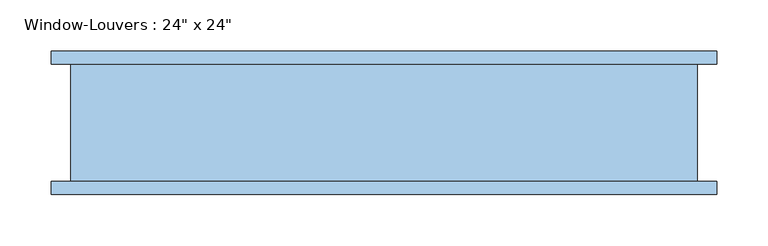
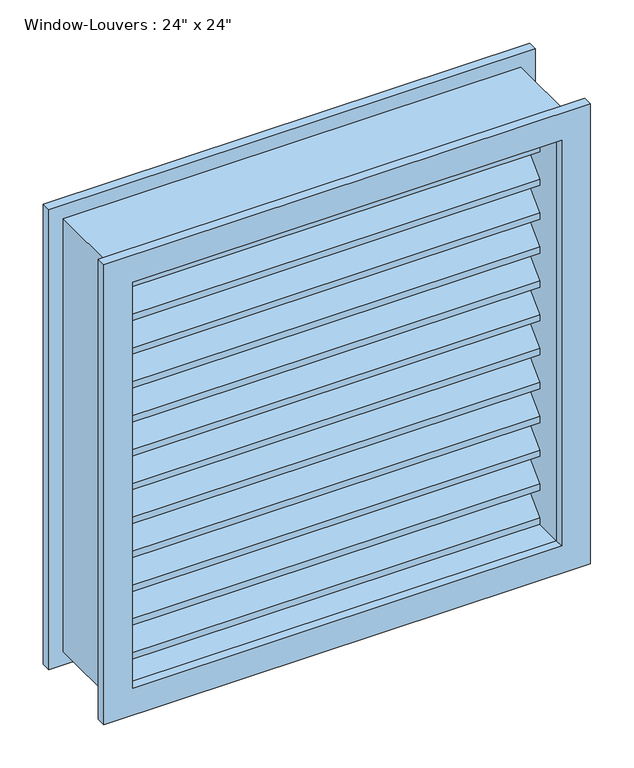
"""IFC4 building model written with IfcOpenShell, lengths in millimetres: window geometry."""

from ifc_helpers import new_model, si_unit, frame, origin, place, context, project, spatial, polyline, outline, extrude, source, transform, mapped, element, save


def window_d39e7ecb(model_context):
    return source(origin(), model_context, "Body", "SweptSolid", [
        extrude(outline(polyline([(50.8, 1419.1754778), (50.8, 1410.1952217), (12.7, 1448.2952217), (-25.4, 1410.1952217), (-25.4, 1419.1754778), (12.7, 1457.2754778), (50.8, 1419.1754778)])), frame((-285.75, 0.0, 0.0), z_axis=(1.0, 0.0, 0.0), x_axis=(0.0, 1.0, 0.0)), (0.0, 0.0, 1.0), 571.5),
        extrude(outline(polyline([(50.8, 1371.5009557), (50.8, 1362.5206995), (12.7, 1400.6206995), (-25.4, 1362.5206995), (-25.4, 1371.5009557), (12.7, 1409.6009557), (50.8, 1371.5009557)])), frame((-285.75, 0.0, 0.0), z_axis=(1.0, 0.0, 0.0), x_axis=(0.0, 1.0, 0.0)), (0.0, 0.0, 1.0), 571.5),
        extrude(outline(polyline([(50.8, 1323.8264335), (50.8, 1314.8461774), (12.7, 1352.9461774), (-25.4, 1314.8461774), (-25.4, 1323.8264335), (12.7, 1361.9264335), (50.8, 1323.8264335)])), frame((-285.75, 0.0, 0.0), z_axis=(1.0, 0.0, 0.0), x_axis=(0.0, 1.0, 0.0)), (0.0, 0.0, 1.0), 571.5),
        extrude(outline(polyline([(50.8, 1276.1519113), (50.8, 1267.1716552), (12.7, 1305.2716552), (-25.4, 1267.1716552), (-25.4, 1276.1519113), (12.7, 1314.2519113), (50.8, 1276.1519113)])), frame((-285.75, 0.0, 0.0), z_axis=(1.0, 0.0, 0.0), x_axis=(0.0, 1.0, 0.0)), (0.0, 0.0, 1.0), 571.5),
        extrude(outline(polyline([(50.8, 1228.4773891), (50.8, 1219.497133), (12.7, 1257.597133), (-25.4, 1219.497133), (-25.4, 1228.4773891), (12.7, 1266.5773891), (50.8, 1228.4773891)])), frame((-285.75, 0.0, 0.0), z_axis=(1.0, 0.0, 0.0), x_axis=(0.0, 1.0, 0.0)), (0.0, 0.0, 1.0), 571.5),
        extrude(outline(polyline([(50.8, 1180.802867), (50.8, 1171.8226109), (12.7, 1209.9226109), (-25.4, 1171.8226109), (-25.4, 1180.802867), (12.7, 1218.902867), (50.8, 1180.802867)])), frame((-285.75, 0.0, 0.0), z_axis=(1.0, 0.0, 0.0), x_axis=(0.0, 1.0, 0.0)), (0.0, 0.0, 1.0), 571.5),
        extrude(outline(polyline([(50.8, 1133.1283448), (50.8, 1124.1480887), (12.7, 1162.2480887), (-25.4, 1124.1480887), (-25.4, 1133.1283448), (12.7, 1171.2283448), (50.8, 1133.1283448)])), frame((-285.75, 0.0, 0.0), z_axis=(1.0, 0.0, 0.0), x_axis=(0.0, 1.0, 0.0)), (0.0, 0.0, 1.0), 571.5),
        extrude(outline(polyline([(50.8, 1085.4538226), (50.8, 1076.4735665), (12.7, 1114.5735665), (-25.4, 1076.4735665), (-25.4, 1085.4538226), (12.7, 1123.5538226), (50.8, 1085.4538226)])), frame((-285.75, 0.0, 0.0), z_axis=(1.0, 0.0, 0.0), x_axis=(0.0, 1.0, 0.0)), (0.0, 0.0, 1.0), 571.5),
        extrude(outline(polyline([(50.8, 1037.7793005), (50.8, 1028.7990443), (12.7, 1066.8990443), (-25.4, 1028.7990443), (-25.4, 1037.7793005), (12.7, 1075.8793005), (50.8, 1037.7793005)])), frame((-285.75, 0.0, 0.0), z_axis=(1.0, 0.0, 0.0), x_axis=(0.0, 1.0, 0.0)), (0.0, 0.0, 1.0), 571.5),
        extrude(outline(polyline([(50.8, 990.1047783), (50.8, 981.1245222), (12.7, 1019.2245222), (-25.4, 981.1245222), (-25.4, 990.1047783), (12.7, 1028.2047783), (50.8, 990.1047783)])), frame((-285.75, 0.0, 0.0), z_axis=(1.0, 0.0, 0.0), x_axis=(0.0, 1.0, 0.0)), (0.0, 0.0, 1.0), 571.5),
        extrude(outline(polyline([(50.8, 1466.85), (50.8, 1457.8697439), (12.7, 1495.9697439), (-25.4, 1457.8697439), (-25.4, 1466.85), (12.7, 1504.95), (50.8, 1466.85)])), frame((-285.75, 0.0, 0.0), z_axis=(1.0, 0.0, 0.0), x_axis=(0.0, 1.0, 0.0)), (0.0, 0.0, 1.0), 571.5),
        extrude(outline(polyline([(50.8, 942.4302561), (50.8, 933.45), (12.7, 971.55), (-25.4, 933.45), (-25.4, 942.4302561), (12.7, 980.5302561), (50.8, 942.4302561)])), frame((-285.75, 0.0, 0.0), z_axis=(1.0, 0.0, 0.0), x_axis=(0.0, 1.0, 0.0)), (0.0, 0.0, 1.0), 571.5),
        extrude(outline(polyline([(1524.0, 304.8), (1524.0, -304.8), (914.4, -304.8), (914.4, 304.8), (1524.0, 304.8)]), holes=[polyline([(1504.95, 285.75), (933.45, 285.75), (933.45, -285.75), (1504.95, -285.75), (1504.95, 285.75)])]), frame((0.0, -63.5, 0.0), z_axis=(0.0, 1.0, 0.0), x_axis=(0.0, 0.0, 1.0)), (0.0, 0.0, 1.0), 114.3),
        extrude(outline(polyline([(1543.05, 323.85), (1543.05, -323.85), (895.35, -323.85), (895.35, 323.85), (1543.05, 323.85)]), holes=[polyline([(1504.95, 285.75), (933.45, 285.75), (933.45, -285.75), (1504.95, -285.75), (1504.95, 285.75)])]), frame((0.0, -76.2, 0.0), z_axis=(0.0, 1.0, 0.0), x_axis=(0.0, 0.0, 1.0)), (0.0, 0.0, 1.0), 12.7),
        extrude(outline(polyline([(1543.05, -323.85), (895.35, -323.85), (895.35, 323.85), (1543.05, 323.85), (1543.05, -323.85)]), holes=[polyline([(1504.95, -285.75), (1504.95, 285.75), (933.45, 285.75), (933.45, -285.75), (1504.95, -285.75)])]), frame((0.0, 50.8, 0.0), z_axis=(0.0, 1.0, 0.0), x_axis=(0.0, 0.0, 1.0)), (0.0, 0.0, 1.0), 12.7),
    ])


if __name__ == "__main__":
    model = new_model("IFC4")
    model_context = context("Model", 3, world=origin())
    ifc_project = project(units=[si_unit("LENGTHUNIT", "METRE", prefix="MILLI")], contexts=[model_context])
    site = spatial("IfcSite", under=ifc_project)
    building = spatial("IfcBuilding", under=site)
    placement = place(None, origin())
    window_shape = window_d39e7ecb(model_context)
    element("IfcWindow", 1, ObjectType="Window-Louvers : 24\" x 24\"", at=placement, inside=building, context=model_context, shape_type="MappedRepresentation", body=[
        mapped(window_shape, transform((0.0, 0.0, 0.0), x_axis=(1.0, 0.0, 0.0), y_axis=(0.0, 1.0, 0.0), z_axis=(0.0, 0.0, 1.0))),
    ])
    save(model, "model.ifc")

# Revit data of these elements
# Type "Window-Louvers : 24\" x 24\""
#   Type Mark = "26"
#   Construction Type Id = "GSP4R"
#   Assembly Code = "B20"
#   Analytic Construction = "1/8 in Pilkington single glazing"
#   Visual Light Transmittance = 0.9
#   Thermal Resistance (R) = 1.53941 (h·ft²·°F)/BTU
#   Solar Heat Gain Coefficient = 0.78
#   Max Height = 1.978553 ft
#   Height = 2 ft
#   Heat Transfer Coefficient (U) = 0.6496 BTU/(h·ft²·°F)
#   Blade Width [instance default] = 1.875 ft
#   Blade Vertical Thickness = 0.029463 ft
#   Blade Thickness = 0.020833 ft
#   Blade Spacing = 0.125 ft
#   Blade Height = 0.154463 ft
#   Blade Depth = 0.25 ft
#   Blade Angle = 45.00°
#   Default Sill Height = 3 ft
#   Trim Projection_Exterior = 0.041667 ft
#   Trim Projection_Interior = 0.041667 ft
#   Trim Width_Exterior = 0.125 ft
#   Trim Width_Interior = 0.125 ft
#   Width = 2 ft
#   Max Blade Count = 12
#   Define Thermal Properties by = 1
#   Blade Count = 12
#   Frame Material = Birch
#   Louver Material = Birch
#   Trim Exterior Material = Birch
#   Trim Interior Material = Birch
#   Wall Closure = (empty or 0)
# Element 1 (IfcWindow, "Window-Louvers : 24\" x 24\"")
#   Materials on its faces: "Birch"
# Materials
#   "Birch": class "Wood", colour RGB 224 178 126, transparency 0, Description = "Betula Alleghaniensis", Cost = 0
